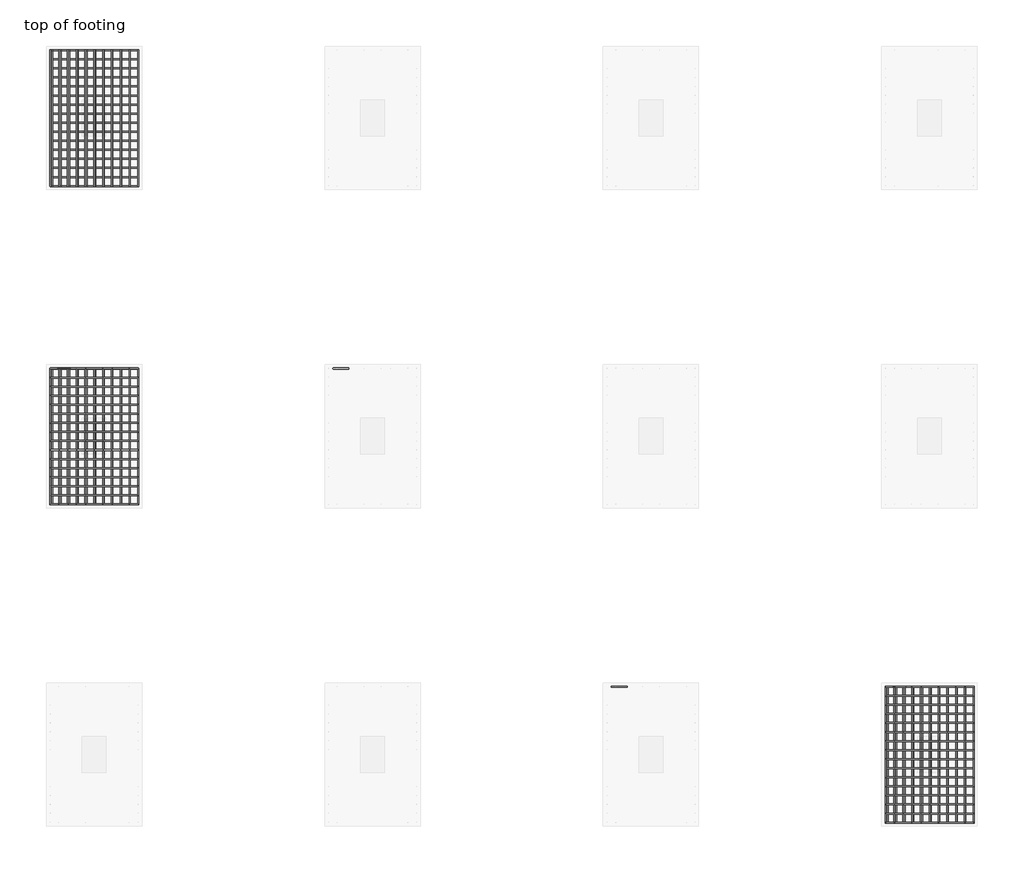
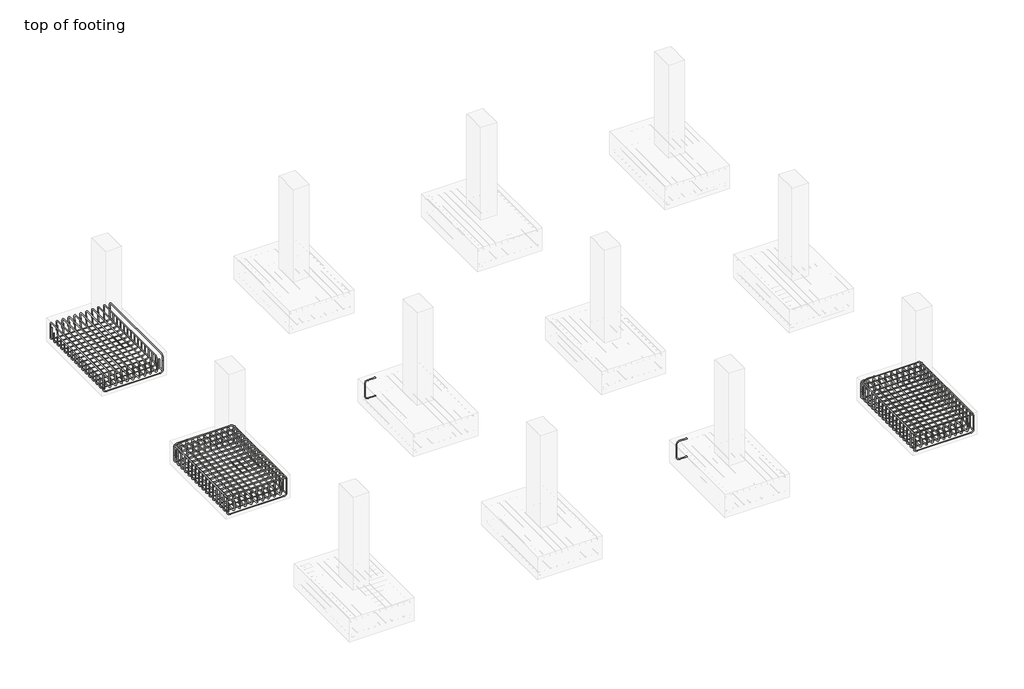
# One storey, part 3 of 8: 15 reinforcing bars.
"""IFC4 building model written with IfcOpenShell, lengths in millimetres."""

from ifc_helpers import new_model, si_unit, point, frame, origin, place, context, project, spatial, polyline, circle_curve, trimmed, segment, composite_curve, source, transform, mapped, element, save
from ifc_brep_helpers import swept_disk

model = new_model("IFC4")

# Units and contexts
model_context = context("Model", 3, world=origin())
ifc_project = project(units=[si_unit("LENGTHUNIT", "METRE", prefix="MILLI")], contexts=[model_context])

# Site, building, storey
site = spatial("IfcSite", under=ifc_project)
building = spatial("IfcBuilding", under=site)
storey = spatial("IfcBuildingStorey", under=building, Name="top of footing", Elevation=-1828.8)

# Reinforcing bars
placement = place(None, origin())
reinforcing_bar_shape = source(origin(), model_context, "Body", "SolidModel", [
    swept_disk(composite_curve([segment(polyline([(-10685.4300189, 12682.8075251, -2014.4920065), (-10685.4300189, 12682.8075251, -2161.7920065)]), True, "CONTINUOUS"), segment(trimmed(circle_curve(frame((-10685.4300189, 12729.1575251, -2161.7920065), z_axis=(1.0, 0.0, 0.0), x_axis=(0.0, -46.350000000000364, 0.0)), 46.35), [point((-10685.4300189, 12682.8075251, -2161.7920065))], [point((-10685.4300189, 12729.1575251, -2208.1420065))], True, "CARTESIAN"), True, "CONTINUOUS"), segment(polyline([(-10685.4300189, 12729.1575251, -2208.1420065), (-10685.4300189, 14343.7575251, -2208.1420065)]), True, "CONTINUOUS"), segment(trimmed(circle_curve(frame((-10685.4300189, 14343.7575251, -2161.7920065), z_axis=(1.0, 0.0, 0.0), x_axis=(0.0, 0.0, -46.350000000000364)), 46.35), [point((-10685.4300189, 14343.7575251, -2208.1420065))], [point((-10685.4300189, 14390.1075251, -2161.7920065))], True, "CARTESIAN"), True, "CONTINUOUS"), segment(polyline([(-10685.4300189, 14390.1075251, -2161.7920065), (-10685.4300189, 14390.1075251, -2014.4920065)]), True, "CONTINUOUS")], self_intersect=False), 6.35),
])
element("IfcReinforcingBar", 1, at=placement, inside=storey, context=model_context, shape_type="MappedRepresentation", body=[
    mapped(reinforcing_bar_shape, transform((0.0, 0.0, 0.0), x_axis=(1.0, 0.0, 0.0), y_axis=(0.0, 1.0, 0.0), z_axis=(0.0, 0.0, 1.0))),
    mapped(reinforcing_bar_shape, transform((-108.3645139, 0.0, 0.0), x_axis=(1.0, 0.0, 0.0), y_axis=(0.0, 1.0, 0.0), z_axis=(0.0, 0.0, 1.0))),
    mapped(reinforcing_bar_shape, transform((-216.7290279, 0.0, 0.0), x_axis=(1.0, 0.0, 0.0), y_axis=(0.0, 1.0, 0.0), z_axis=(0.0, 0.0, 1.0))),
    mapped(reinforcing_bar_shape, transform((-325.0935418, 0.0, 0.0), x_axis=(1.0, 0.0, 0.0), y_axis=(0.0, 1.0, 0.0), z_axis=(0.0, 0.0, 1.0))),
    mapped(reinforcing_bar_shape, transform((-433.4580557, 0.0, 0.0), x_axis=(1.0, 0.0, 0.0), y_axis=(0.0, 1.0, 0.0), z_axis=(0.0, 0.0, 1.0))),
    mapped(reinforcing_bar_shape, transform((-541.8225696, 0.0, 0.0), x_axis=(1.0, 0.0, 0.0), y_axis=(0.0, 1.0, 0.0), z_axis=(0.0, 0.0, 1.0))),
    mapped(reinforcing_bar_shape, transform((-650.1870836, 0.0, 0.0), x_axis=(1.0, 0.0, 0.0), y_axis=(0.0, 1.0, 0.0), z_axis=(0.0, 0.0, 1.0))),
    mapped(reinforcing_bar_shape, transform((-758.5515975, 0.0, 0.0), x_axis=(1.0, 0.0, 0.0), y_axis=(0.0, 1.0, 0.0), z_axis=(0.0, 0.0, 1.0))),
    mapped(reinforcing_bar_shape, transform((-866.9161114, 0.0, 0.0), x_axis=(1.0, 0.0, 0.0), y_axis=(0.0, 1.0, 0.0), z_axis=(0.0, 0.0, 1.0))),
    mapped(reinforcing_bar_shape, transform((-975.2806253, 0.0, 0.0), x_axis=(1.0, 0.0, 0.0), y_axis=(0.0, 1.0, 0.0), z_axis=(0.0, 0.0, 1.0))),
    mapped(reinforcing_bar_shape, transform((-1083.6451393, 0.0, 0.0), x_axis=(1.0, 0.0, 0.0), y_axis=(0.0, 1.0, 0.0), z_axis=(0.0, 0.0, 1.0))),
])
reinforcing_bar_2_shape = source(origin(), model_context, "Body", "SolidModel", [
    swept_disk(composite_curve([segment(polyline([(-11792.7300189, 12682.8075251, -2085.8010212), (-11792.7300189, 12682.8075251, -1938.5010212)]), True, "CONTINUOUS"), segment(trimmed(circle_curve(frame((-11792.7300189, 12729.1575251, -1938.5010212), z_axis=(-1.0, 0.0, 0.0), x_axis=(0.0, -46.350000000000364, 0.0)), 46.35), [point((-11792.7300189, 12682.8075251, -1938.5010212))], [point((-11792.7300189, 12729.1575251, -1892.1510212))], True, "CARTESIAN"), True, "CONTINUOUS"), segment(polyline([(-11792.7300189, 12729.1575251, -1892.1510212), (-11792.7300189, 14343.7575251, -1892.1510212)]), True, "CONTINUOUS"), segment(trimmed(circle_curve(frame((-11792.7300189, 14343.7575251, -1938.5010212), z_axis=(-1.0, 0.0, 0.0), x_axis=(0.0, 0.0, 46.34999999999991)), 46.35), [point((-11792.7300189, 14343.7575251, -1892.1510212))], [point((-11792.7300189, 14390.1075251, -1938.5010212))], True, "CARTESIAN"), True, "CONTINUOUS"), segment(polyline([(-11792.7300189, 14390.1075251, -1938.5010212), (-11792.7300189, 14390.1075251, -2085.8010212)]), True, "CONTINUOUS")], self_intersect=False), 6.35),
])
element("IfcReinforcingBar", 2, at=placement, inside=storey, context=model_context, shape_type="MappedRepresentation", body=[
    mapped(reinforcing_bar_2_shape, transform((0.0, 0.0, 0.0), x_axis=(1.0, 0.0, 0.0), y_axis=(0.0, 1.0, 0.0), z_axis=(0.0, 0.0, 1.0))),
    mapped(reinforcing_bar_2_shape, transform((110.73, 0.0, 0.0), x_axis=(1.0, 0.0, 0.0), y_axis=(0.0, 1.0, 0.0), z_axis=(0.0, 0.0, 1.0))),
    mapped(reinforcing_bar_2_shape, transform((221.46, 0.0, 0.0), x_axis=(1.0, 0.0, 0.0), y_axis=(0.0, 1.0, 0.0), z_axis=(0.0, 0.0, 1.0))),
    mapped(reinforcing_bar_2_shape, transform((332.19, 0.0, 0.0), x_axis=(1.0, 0.0, 0.0), y_axis=(0.0, 1.0, 0.0), z_axis=(0.0, 0.0, 1.0))),
    mapped(reinforcing_bar_2_shape, transform((442.92, 0.0, 0.0), x_axis=(1.0, 0.0, 0.0), y_axis=(0.0, 1.0, 0.0), z_axis=(0.0, 0.0, 1.0))),
    mapped(reinforcing_bar_2_shape, transform((553.65, 0.0, 0.0), x_axis=(1.0, 0.0, 0.0), y_axis=(0.0, 1.0, 0.0), z_axis=(0.0, 0.0, 1.0))),
    mapped(reinforcing_bar_2_shape, transform((664.38, 0.0, 0.0), x_axis=(1.0, 0.0, 0.0), y_axis=(0.0, 1.0, 0.0), z_axis=(0.0, 0.0, 1.0))),
    mapped(reinforcing_bar_2_shape, transform((775.11, 0.0, 0.0), x_axis=(1.0, 0.0, 0.0), y_axis=(0.0, 1.0, 0.0), z_axis=(0.0, 0.0, 1.0))),
    mapped(reinforcing_bar_2_shape, transform((885.84, 0.0, 0.0), x_axis=(1.0, 0.0, 0.0), y_axis=(0.0, 1.0, 0.0), z_axis=(0.0, 0.0, 1.0))),
    mapped(reinforcing_bar_2_shape, transform((996.57, 0.0, 0.0), x_axis=(1.0, 0.0, 0.0), y_axis=(0.0, 1.0, 0.0), z_axis=(0.0, 0.0, 1.0))),
    mapped(reinforcing_bar_2_shape, transform((1107.3, 0.0, 0.0), x_axis=(1.0, 0.0, 0.0), y_axis=(0.0, 1.0, 0.0), z_axis=(0.0, 0.0, 1.0))),
])
reinforcing_bar_3_shape = source(origin(), model_context, "Body", "SolidModel", [
    swept_disk(composite_curve([segment(polyline([(-10685.4300189, 14390.1075251, -2044.8290141), (-10685.4300189, 14390.1075251, -2192.1290141)]), True, "CONTINUOUS"), segment(trimmed(circle_curve(frame((-10731.7800189, 14390.1075251, -2192.1290141), z_axis=(0.0, 1.0, 0.0), x_axis=(46.350000000000364, 0.0, 0.0)), 46.35), [point((-10685.4300189, 14390.1075251, -2192.1290141))], [point((-10731.7800189, 14390.1075251, -2238.4790141))], True, "CARTESIAN"), True, "CONTINUOUS"), segment(polyline([(-10731.7800189, 14390.1075251, -2238.4790141), (-11746.3800189, 14390.1075251, -2238.4790141)]), True, "CONTINUOUS"), segment(trimmed(circle_curve(frame((-11746.3800189, 14390.1075251, -2192.1290141), z_axis=(0.0, 1.0, 0.0), x_axis=(0.0, 0.0, -46.34999999999991)), 46.35), [point((-11746.3800189, 14390.1075251, -2238.4790141))], [point((-11792.7300189, 14390.1075251, -2192.1290141))], True, "CARTESIAN"), True, "CONTINUOUS"), segment(polyline([(-11792.7300189, 14390.1075251, -2192.1290141), (-11792.7300189, 14390.1075251, -2044.8290141)]), True, "CONTINUOUS")], self_intersect=False), 6.35),
])
element("IfcReinforcingBar", 3, at=placement, inside=storey, context=model_context, shape_type="MappedRepresentation", body=[
    mapped(reinforcing_bar_3_shape, transform((0.0, 0.0, 0.0), x_axis=(1.0, 0.0, 0.0), y_axis=(0.0, 1.0, 0.0), z_axis=(0.0, 0.0, 1.0))),
    mapped(reinforcing_bar_3_shape, transform((0.0, -113.82, 0.0), x_axis=(1.0, 0.0, 0.0), y_axis=(0.0, 1.0, 0.0), z_axis=(0.0, 0.0, 1.0))),
    mapped(reinforcing_bar_3_shape, transform((0.0, -227.64, 0.0), x_axis=(1.0, 0.0, 0.0), y_axis=(0.0, 1.0, 0.0), z_axis=(0.0, 0.0, 1.0))),
    mapped(reinforcing_bar_3_shape, transform((0.0, -341.46, 0.0), x_axis=(1.0, 0.0, 0.0), y_axis=(0.0, 1.0, 0.0), z_axis=(0.0, 0.0, 1.0))),
    mapped(reinforcing_bar_3_shape, transform((0.0, -455.28, 0.0), x_axis=(1.0, 0.0, 0.0), y_axis=(0.0, 1.0, 0.0), z_axis=(0.0, 0.0, 1.0))),
    mapped(reinforcing_bar_3_shape, transform((0.0, -569.1, 0.0), x_axis=(1.0, 0.0, 0.0), y_axis=(0.0, 1.0, 0.0), z_axis=(0.0, 0.0, 1.0))),
    mapped(reinforcing_bar_3_shape, transform((0.0, -682.92, 0.0), x_axis=(1.0, 0.0, 0.0), y_axis=(0.0, 1.0, 0.0), z_axis=(0.0, 0.0, 1.0))),
    mapped(reinforcing_bar_3_shape, transform((0.0, -796.74, 0.0), x_axis=(1.0, 0.0, 0.0), y_axis=(0.0, 1.0, 0.0), z_axis=(0.0, 0.0, 1.0))),
    mapped(reinforcing_bar_3_shape, transform((0.0, -910.56, 0.0), x_axis=(1.0, 0.0, 0.0), y_axis=(0.0, 1.0, 0.0), z_axis=(0.0, 0.0, 1.0))),
    mapped(reinforcing_bar_3_shape, transform((0.0, -1024.38, 0.0), x_axis=(1.0, 0.0, 0.0), y_axis=(0.0, 1.0, 0.0), z_axis=(0.0, 0.0, 1.0))),
    mapped(reinforcing_bar_3_shape, transform((0.0, -1138.2, 0.0), x_axis=(1.0, 0.0, 0.0), y_axis=(0.0, 1.0, 0.0), z_axis=(0.0, 0.0, 1.0))),
    mapped(reinforcing_bar_3_shape, transform((0.0, -1252.02, 0.0), x_axis=(1.0, 0.0, 0.0), y_axis=(0.0, 1.0, 0.0), z_axis=(0.0, 0.0, 1.0))),
    mapped(reinforcing_bar_3_shape, transform((0.0, -1365.84, 0.0), x_axis=(1.0, 0.0, 0.0), y_axis=(0.0, 1.0, 0.0), z_axis=(0.0, 0.0, 1.0))),
    mapped(reinforcing_bar_3_shape, transform((0.0, -1479.66, 0.0), x_axis=(1.0, 0.0, 0.0), y_axis=(0.0, 1.0, 0.0), z_axis=(0.0, 0.0, 1.0))),
    mapped(reinforcing_bar_3_shape, transform((0.0, -1593.48, 0.0), x_axis=(1.0, 0.0, 0.0), y_axis=(0.0, 1.0, 0.0), z_axis=(0.0, 0.0, 1.0))),
    mapped(reinforcing_bar_3_shape, transform((0.0, -1707.3, 0.0), x_axis=(1.0, 0.0, 0.0), y_axis=(0.0, 1.0, 0.0), z_axis=(0.0, 0.0, 1.0))),
])
reinforcing_bar_4_shape = source(origin(), model_context, "Body", "SolidModel", [
    swept_disk(composite_curve([segment(polyline([(-10685.4300189, 8682.8075251, -2014.4920065), (-10685.4300189, 8682.8075251, -2161.7920065)]), True, "CONTINUOUS"), segment(trimmed(circle_curve(frame((-10685.4300189, 8729.1575251, -2161.7920065), z_axis=(1.0, 0.0, 0.0), x_axis=(0.0, -46.350000000000364, 0.0)), 46.35), [point((-10685.4300189, 8682.8075251, -2161.7920065))], [point((-10685.4300189, 8729.1575251, -2208.1420065))], True, "CARTESIAN"), True, "CONTINUOUS"), segment(polyline([(-10685.4300189, 8729.1575251, -2208.1420065), (-10685.4300189, 10343.7575251, -2208.1420065)]), True, "CONTINUOUS"), segment(trimmed(circle_curve(frame((-10685.4300189, 10343.7575251, -2161.7920065), z_axis=(1.0, 0.0, 0.0), x_axis=(0.0, 0.0, -46.350000000000364)), 46.35), [point((-10685.4300189, 10343.7575251, -2208.1420065))], [point((-10685.4300189, 10390.1075251, -2161.7920065))], True, "CARTESIAN"), True, "CONTINUOUS"), segment(polyline([(-10685.4300189, 10390.1075251, -2161.7920065), (-10685.4300189, 10390.1075251, -2014.4920065)]), True, "CONTINUOUS")], self_intersect=False), 6.35),
])
element("IfcReinforcingBar", 4, at=placement, inside=storey, context=model_context, shape_type="MappedRepresentation", body=[
    mapped(reinforcing_bar_4_shape, transform((0.0, 0.0, 0.0), x_axis=(1.0, 0.0, 0.0), y_axis=(0.0, 1.0, 0.0), z_axis=(0.0, 0.0, 1.0))),
    mapped(reinforcing_bar_4_shape, transform((-108.3645139, 0.0, 0.0), x_axis=(1.0, 0.0, 0.0), y_axis=(0.0, 1.0, 0.0), z_axis=(0.0, 0.0, 1.0))),
    mapped(reinforcing_bar_4_shape, transform((-216.7290279, 0.0, 0.0), x_axis=(1.0, 0.0, 0.0), y_axis=(0.0, 1.0, 0.0), z_axis=(0.0, 0.0, 1.0))),
    mapped(reinforcing_bar_4_shape, transform((-325.0935418, 0.0, 0.0), x_axis=(1.0, 0.0, 0.0), y_axis=(0.0, 1.0, 0.0), z_axis=(0.0, 0.0, 1.0))),
    mapped(reinforcing_bar_4_shape, transform((-433.4580557, 0.0, 0.0), x_axis=(1.0, 0.0, 0.0), y_axis=(0.0, 1.0, 0.0), z_axis=(0.0, 0.0, 1.0))),
    mapped(reinforcing_bar_4_shape, transform((-541.8225696, 0.0, 0.0), x_axis=(1.0, 0.0, 0.0), y_axis=(0.0, 1.0, 0.0), z_axis=(0.0, 0.0, 1.0))),
    mapped(reinforcing_bar_4_shape, transform((-650.1870836, 0.0, 0.0), x_axis=(1.0, 0.0, 0.0), y_axis=(0.0, 1.0, 0.0), z_axis=(0.0, 0.0, 1.0))),
    mapped(reinforcing_bar_4_shape, transform((-758.5515975, 0.0, 0.0), x_axis=(1.0, 0.0, 0.0), y_axis=(0.0, 1.0, 0.0), z_axis=(0.0, 0.0, 1.0))),
    mapped(reinforcing_bar_4_shape, transform((-866.9161114, 0.0, 0.0), x_axis=(1.0, 0.0, 0.0), y_axis=(0.0, 1.0, 0.0), z_axis=(0.0, 0.0, 1.0))),
    mapped(reinforcing_bar_4_shape, transform((-975.2806253, 0.0, 0.0), x_axis=(1.0, 0.0, 0.0), y_axis=(0.0, 1.0, 0.0), z_axis=(0.0, 0.0, 1.0))),
    mapped(reinforcing_bar_4_shape, transform((-1083.6451393, 0.0, 0.0), x_axis=(1.0, 0.0, 0.0), y_axis=(0.0, 1.0, 0.0), z_axis=(0.0, 0.0, 1.0))),
])
reinforcing_bar_5_shape = source(origin(), model_context, "Body", "SolidModel", [
    swept_disk(composite_curve([segment(polyline([(-11792.7300189, 8682.8075251, -2085.8010212), (-11792.7300189, 8682.8075251, -1938.5010212)]), True, "CONTINUOUS"), segment(trimmed(circle_curve(frame((-11792.7300189, 8729.1575251, -1938.5010212), z_axis=(-1.0, 0.0, 0.0), x_axis=(0.0, -46.350000000000364, 0.0)), 46.35), [point((-11792.7300189, 8682.8075251, -1938.5010212))], [point((-11792.7300189, 8729.1575251, -1892.1510212))], True, "CARTESIAN"), True, "CONTINUOUS"), segment(polyline([(-11792.7300189, 8729.1575251, -1892.1510212), (-11792.7300189, 10343.7575251, -1892.1510212)]), True, "CONTINUOUS"), segment(trimmed(circle_curve(frame((-11792.7300189, 10343.7575251, -1938.5010212), z_axis=(-1.0, 0.0, 0.0), x_axis=(0.0, 0.0, 46.34999999999991)), 46.35), [point((-11792.7300189, 10343.7575251, -1892.1510212))], [point((-11792.7300189, 10390.1075251, -1938.5010212))], True, "CARTESIAN"), True, "CONTINUOUS"), segment(polyline([(-11792.7300189, 10390.1075251, -1938.5010212), (-11792.7300189, 10390.1075251, -2085.8010212)]), True, "CONTINUOUS")], self_intersect=False), 6.35),
])
element("IfcReinforcingBar", 5, at=placement, inside=storey, context=model_context, shape_type="MappedRepresentation", body=[
    mapped(reinforcing_bar_5_shape, transform((0.0, 0.0, 0.0), x_axis=(1.0, 0.0, 0.0), y_axis=(0.0, 1.0, 0.0), z_axis=(0.0, 0.0, 1.0))),
    mapped(reinforcing_bar_5_shape, transform((110.73, 0.0, 0.0), x_axis=(1.0, 0.0, 0.0), y_axis=(0.0, 1.0, 0.0), z_axis=(0.0, 0.0, 1.0))),
    mapped(reinforcing_bar_5_shape, transform((221.46, 0.0, 0.0), x_axis=(1.0, 0.0, 0.0), y_axis=(0.0, 1.0, 0.0), z_axis=(0.0, 0.0, 1.0))),
    mapped(reinforcing_bar_5_shape, transform((332.19, 0.0, 0.0), x_axis=(1.0, 0.0, 0.0), y_axis=(0.0, 1.0, 0.0), z_axis=(0.0, 0.0, 1.0))),
    mapped(reinforcing_bar_5_shape, transform((442.92, 0.0, 0.0), x_axis=(1.0, 0.0, 0.0), y_axis=(0.0, 1.0, 0.0), z_axis=(0.0, 0.0, 1.0))),
    mapped(reinforcing_bar_5_shape, transform((553.65, 0.0, 0.0), x_axis=(1.0, 0.0, 0.0), y_axis=(0.0, 1.0, 0.0), z_axis=(0.0, 0.0, 1.0))),
    mapped(reinforcing_bar_5_shape, transform((664.38, 0.0, 0.0), x_axis=(1.0, 0.0, 0.0), y_axis=(0.0, 1.0, 0.0), z_axis=(0.0, 0.0, 1.0))),
    mapped(reinforcing_bar_5_shape, transform((775.11, 0.0, 0.0), x_axis=(1.0, 0.0, 0.0), y_axis=(0.0, 1.0, 0.0), z_axis=(0.0, 0.0, 1.0))),
    mapped(reinforcing_bar_5_shape, transform((885.84, 0.0, 0.0), x_axis=(1.0, 0.0, 0.0), y_axis=(0.0, 1.0, 0.0), z_axis=(0.0, 0.0, 1.0))),
    mapped(reinforcing_bar_5_shape, transform((996.57, 0.0, 0.0), x_axis=(1.0, 0.0, 0.0), y_axis=(0.0, 1.0, 0.0), z_axis=(0.0, 0.0, 1.0))),
    mapped(reinforcing_bar_5_shape, transform((1107.3, 0.0, 0.0), x_axis=(1.0, 0.0, 0.0), y_axis=(0.0, 1.0, 0.0), z_axis=(0.0, 0.0, 1.0))),
])
element("IfcReinforcingBar", 6, at=placement, inside=storey, context=model_context, shape_type="SolidModel", body=[
    swept_disk(composite_curve([segment(polyline([(-11543.0309105, 10390.1075251, -2232.45), (-11690.3309105, 10390.1075251, -2232.45)]), True, "CONTINUOUS"), segment(trimmed(circle_curve(frame((-11690.3309105, 10390.1075251, -2186.1), z_axis=(0.0, 1.0, 0.0), x_axis=(0.0, 0.0, -46.34999999999991)), 46.35), [point((-11690.3309105, 10390.1075251, -2232.45))], [point((-11736.6809105, 10390.1075251, -2186.1))], True, "CARTESIAN"), True, "CONTINUOUS"), segment(polyline([(-11736.6809105, 10390.1075251, -2186.1), (-11736.6809105, 10390.1075251, -1921.5)]), True, "CONTINUOUS"), segment(trimmed(circle_curve(frame((-11690.3309105, 10390.1075251, -1921.5), z_axis=(0.0, 1.0, 0.0), x_axis=(-46.349999999998545, 0.0, 0.0)), 46.35), [point((-11736.6809105, 10390.1075251, -1921.5))], [point((-11690.3309105, 10390.1075251, -1875.15))], True, "CARTESIAN"), True, "CONTINUOUS"), segment(polyline([(-11690.3309105, 10390.1075251, -1875.15), (-11543.0309105, 10390.1075251, -1875.15)]), True, "CONTINUOUS")], self_intersect=False), 6.35),
])
reinforcing_bar_6_shape = source(origin(), model_context, "Body", "SolidModel", [
    swept_disk(composite_curve([segment(polyline([(-10685.4300189, 10390.1075251, -2044.8290141), (-10685.4300189, 10390.1075251, -2192.1290141)]), True, "CONTINUOUS"), segment(trimmed(circle_curve(frame((-10731.7800189, 10390.1075251, -2192.1290141), z_axis=(0.0, 1.0, 0.0), x_axis=(46.350000000000364, 0.0, 0.0)), 46.35), [point((-10685.4300189, 10390.1075251, -2192.1290141))], [point((-10731.7800189, 10390.1075251, -2238.4790141))], True, "CARTESIAN"), True, "CONTINUOUS"), segment(polyline([(-10731.7800189, 10390.1075251, -2238.4790141), (-11746.3800189, 10390.1075251, -2238.4790141)]), True, "CONTINUOUS"), segment(trimmed(circle_curve(frame((-11746.3800189, 10390.1075251, -2192.1290141), z_axis=(0.0, 1.0, 0.0), x_axis=(0.0, 0.0, -46.34999999999991)), 46.35), [point((-11746.3800189, 10390.1075251, -2238.4790141))], [point((-11792.7300189, 10390.1075251, -2192.1290141))], True, "CARTESIAN"), True, "CONTINUOUS"), segment(polyline([(-11792.7300189, 10390.1075251, -2192.1290141), (-11792.7300189, 10390.1075251, -2044.8290141)]), True, "CONTINUOUS")], self_intersect=False), 6.35),
])
element("IfcReinforcingBar", 7, at=placement, inside=storey, context=model_context, shape_type="MappedRepresentation", body=[
    mapped(reinforcing_bar_6_shape, transform((0.0, 0.0, 0.0), x_axis=(1.0, 0.0, 0.0), y_axis=(0.0, 1.0, 0.0), z_axis=(0.0, 0.0, 1.0))),
    mapped(reinforcing_bar_6_shape, transform((0.0, -113.82, 0.0), x_axis=(1.0, 0.0, 0.0), y_axis=(0.0, 1.0, 0.0), z_axis=(0.0, 0.0, 1.0))),
    mapped(reinforcing_bar_6_shape, transform((0.0, -227.64, 0.0), x_axis=(1.0, 0.0, 0.0), y_axis=(0.0, 1.0, 0.0), z_axis=(0.0, 0.0, 1.0))),
    mapped(reinforcing_bar_6_shape, transform((0.0, -341.46, 0.0), x_axis=(1.0, 0.0, 0.0), y_axis=(0.0, 1.0, 0.0), z_axis=(0.0, 0.0, 1.0))),
    mapped(reinforcing_bar_6_shape, transform((0.0, -455.28, 0.0), x_axis=(1.0, 0.0, 0.0), y_axis=(0.0, 1.0, 0.0), z_axis=(0.0, 0.0, 1.0))),
    mapped(reinforcing_bar_6_shape, transform((0.0, -569.1, 0.0), x_axis=(1.0, 0.0, 0.0), y_axis=(0.0, 1.0, 0.0), z_axis=(0.0, 0.0, 1.0))),
    mapped(reinforcing_bar_6_shape, transform((0.0, -682.92, 0.0), x_axis=(1.0, 0.0, 0.0), y_axis=(0.0, 1.0, 0.0), z_axis=(0.0, 0.0, 1.0))),
    mapped(reinforcing_bar_6_shape, transform((0.0, -796.74, 0.0), x_axis=(1.0, 0.0, 0.0), y_axis=(0.0, 1.0, 0.0), z_axis=(0.0, 0.0, 1.0))),
    mapped(reinforcing_bar_6_shape, transform((0.0, -910.56, 0.0), x_axis=(1.0, 0.0, 0.0), y_axis=(0.0, 1.0, 0.0), z_axis=(0.0, 0.0, 1.0))),
    mapped(reinforcing_bar_6_shape, transform((0.0, -1024.38, 0.0), x_axis=(1.0, 0.0, 0.0), y_axis=(0.0, 1.0, 0.0), z_axis=(0.0, 0.0, 1.0))),
    mapped(reinforcing_bar_6_shape, transform((0.0, -1138.2, 0.0), x_axis=(1.0, 0.0, 0.0), y_axis=(0.0, 1.0, 0.0), z_axis=(0.0, 0.0, 1.0))),
    mapped(reinforcing_bar_6_shape, transform((0.0, -1252.02, 0.0), x_axis=(1.0, 0.0, 0.0), y_axis=(0.0, 1.0, 0.0), z_axis=(0.0, 0.0, 1.0))),
    mapped(reinforcing_bar_6_shape, transform((0.0, -1365.84, 0.0), x_axis=(1.0, 0.0, 0.0), y_axis=(0.0, 1.0, 0.0), z_axis=(0.0, 0.0, 1.0))),
    mapped(reinforcing_bar_6_shape, transform((0.0, -1479.66, 0.0), x_axis=(1.0, 0.0, 0.0), y_axis=(0.0, 1.0, 0.0), z_axis=(0.0, 0.0, 1.0))),
    mapped(reinforcing_bar_6_shape, transform((0.0, -1593.48, 0.0), x_axis=(1.0, 0.0, 0.0), y_axis=(0.0, 1.0, 0.0), z_axis=(0.0, 0.0, 1.0))),
    mapped(reinforcing_bar_6_shape, transform((0.0, -1707.3, 0.0), x_axis=(1.0, 0.0, 0.0), y_axis=(0.0, 1.0, 0.0), z_axis=(0.0, 0.0, 1.0))),
])
reinforcing_bar_7_shape = source(origin(), model_context, "Body", "SolidModel", [
    swept_disk(composite_curve([segment(polyline([(-11792.7300189, 10390.1075251, -2075.0801535), (-11792.7300189, 10390.1075251, -1927.7801535)]), True, "CONTINUOUS"), segment(trimmed(circle_curve(frame((-11746.3800189, 10390.1075251, -1927.7801535), z_axis=(0.0, 1.0, 0.0), x_axis=(-46.350000000000364, 0.0, 0.0)), 46.35), [point((-11792.7300189, 10390.1075251, -1927.7801535))], [point((-11746.3800189, 10390.1075251, -1881.4301535))], True, "CARTESIAN"), True, "CONTINUOUS"), segment(polyline([(-11746.3800189, 10390.1075251, -1881.4301535), (-10731.7800189, 10390.1075251, -1881.4301535)]), True, "CONTINUOUS"), segment(trimmed(circle_curve(frame((-10731.7800189, 10390.1075251, -1927.7801535), z_axis=(0.0, 1.0, 0.0), x_axis=(0.0, 0.0, 46.350000000000136)), 46.35), [point((-10731.7800189, 10390.1075251, -1881.4301535))], [point((-10685.4300189, 10390.1075251, -1927.7801535))], True, "CARTESIAN"), True, "CONTINUOUS"), segment(polyline([(-10685.4300189, 10390.1075251, -1927.7801535), (-10685.4300189, 10390.1075251, -2075.0801535)]), True, "CONTINUOUS")], self_intersect=False), 6.35),
])
element("IfcReinforcingBar", 8, at=placement, inside=storey, context=model_context, shape_type="MappedRepresentation", body=[
    mapped(reinforcing_bar_7_shape, transform((0.0, 0.0, 0.0), x_axis=(1.0, 0.0, 0.0), y_axis=(0.0, 1.0, 0.0), z_axis=(0.0, 0.0, 1.0))),
    mapped(reinforcing_bar_7_shape, transform((0.0, -113.82, 0.0), x_axis=(1.0, 0.0, 0.0), y_axis=(0.0, 1.0, 0.0), z_axis=(0.0, 0.0, 1.0))),
    mapped(reinforcing_bar_7_shape, transform((0.0, -227.64, 0.0), x_axis=(1.0, 0.0, 0.0), y_axis=(0.0, 1.0, 0.0), z_axis=(0.0, 0.0, 1.0))),
    mapped(reinforcing_bar_7_shape, transform((0.0, -341.46, 0.0), x_axis=(1.0, 0.0, 0.0), y_axis=(0.0, 1.0, 0.0), z_axis=(0.0, 0.0, 1.0))),
    mapped(reinforcing_bar_7_shape, transform((0.0, -455.28, 0.0), x_axis=(1.0, 0.0, 0.0), y_axis=(0.0, 1.0, 0.0), z_axis=(0.0, 0.0, 1.0))),
    mapped(reinforcing_bar_7_shape, transform((0.0, -569.1, 0.0), x_axis=(1.0, 0.0, 0.0), y_axis=(0.0, 1.0, 0.0), z_axis=(0.0, 0.0, 1.0))),
    mapped(reinforcing_bar_7_shape, transform((0.0, -682.92, 0.0), x_axis=(1.0, 0.0, 0.0), y_axis=(0.0, 1.0, 0.0), z_axis=(0.0, 0.0, 1.0))),
    mapped(reinforcing_bar_7_shape, transform((0.0, -796.74, 0.0), x_axis=(1.0, 0.0, 0.0), y_axis=(0.0, 1.0, 0.0), z_axis=(0.0, 0.0, 1.0))),
    mapped(reinforcing_bar_7_shape, transform((0.0, -910.56, 0.0), x_axis=(1.0, 0.0, 0.0), y_axis=(0.0, 1.0, 0.0), z_axis=(0.0, 0.0, 1.0))),
    mapped(reinforcing_bar_7_shape, transform((0.0, -1024.38, 0.0), x_axis=(1.0, 0.0, 0.0), y_axis=(0.0, 1.0, 0.0), z_axis=(0.0, 0.0, 1.0))),
    mapped(reinforcing_bar_7_shape, transform((0.0, -1138.2, 0.0), x_axis=(1.0, 0.0, 0.0), y_axis=(0.0, 1.0, 0.0), z_axis=(0.0, 0.0, 1.0))),
    mapped(reinforcing_bar_7_shape, transform((0.0, -1252.02, 0.0), x_axis=(1.0, 0.0, 0.0), y_axis=(0.0, 1.0, 0.0), z_axis=(0.0, 0.0, 1.0))),
    mapped(reinforcing_bar_7_shape, transform((0.0, -1365.84, 0.0), x_axis=(1.0, 0.0, 0.0), y_axis=(0.0, 1.0, 0.0), z_axis=(0.0, 0.0, 1.0))),
    mapped(reinforcing_bar_7_shape, transform((0.0, -1479.66, 0.0), x_axis=(1.0, 0.0, 0.0), y_axis=(0.0, 1.0, 0.0), z_axis=(0.0, 0.0, 1.0))),
    mapped(reinforcing_bar_7_shape, transform((0.0, -1593.48, 0.0), x_axis=(1.0, 0.0, 0.0), y_axis=(0.0, 1.0, 0.0), z_axis=(0.0, 0.0, 1.0))),
    mapped(reinforcing_bar_7_shape, transform((0.0, -1707.3, 0.0), x_axis=(1.0, 0.0, 0.0), y_axis=(0.0, 1.0, 0.0), z_axis=(0.0, 0.0, 1.0))),
])
element("IfcReinforcingBar", 9, at=placement, inside=storey, context=model_context, shape_type="SolidModel", body=[
    swept_disk(composite_curve([segment(polyline([(-4543.0309105, 6390.1075251, -2232.45), (-4690.3309105, 6390.1075251, -2232.45)]), True, "CONTINUOUS"), segment(trimmed(circle_curve(frame((-4690.3309105, 6390.1075251, -2186.1), z_axis=(0.0, 1.0, 0.0), x_axis=(0.0, 0.0, -46.34999999999991)), 46.35), [point((-4690.3309105, 6390.1075251, -2232.45))], [point((-4736.6809105, 6390.1075251, -2186.1))], True, "CARTESIAN"), True, "CONTINUOUS"), segment(polyline([(-4736.6809105, 6390.1075251, -2186.1), (-4736.6809105, 6390.1075251, -1921.5)]), True, "CONTINUOUS"), segment(trimmed(circle_curve(frame((-4690.3309105, 6390.1075251, -1921.5), z_axis=(0.0, 1.0, 0.0), x_axis=(-46.350000000000364, 0.0, 0.0)), 46.35), [point((-4736.6809105, 6390.1075251, -1921.5))], [point((-4690.3309105, 6390.1075251, -1875.15))], True, "CARTESIAN"), True, "CONTINUOUS"), segment(polyline([(-4690.3309105, 6390.1075251, -1875.15), (-4543.0309105, 6390.1075251, -1875.15)]), True, "CONTINUOUS")], self_intersect=False), 6.35),
])
reinforcing_bar_8_shape = source(origin(), model_context, "Body", "SolidModel", [
    swept_disk(composite_curve([segment(polyline([(-185.4300189, 4682.8075251, -2014.4920065), (-185.4300189, 4682.8075251, -2161.7920065)]), True, "CONTINUOUS"), segment(trimmed(circle_curve(frame((-185.4300189, 4729.1575251, -2161.7920065), z_axis=(1.0, 0.0, 0.0), x_axis=(0.0, -46.350000000000364, 0.0)), 46.35), [point((-185.4300189, 4682.8075251, -2161.7920065))], [point((-185.4300189, 4729.1575251, -2208.1420065))], True, "CARTESIAN"), True, "CONTINUOUS"), segment(polyline([(-185.4300189, 4729.1575251, -2208.1420065), (-185.4300189, 6343.7575251, -2208.1420065)]), True, "CONTINUOUS"), segment(trimmed(circle_curve(frame((-185.4300189, 6343.7575251, -2161.7920065), z_axis=(1.0, 0.0, 0.0), x_axis=(0.0, 0.0, -46.350000000000364)), 46.35), [point((-185.4300189, 6343.7575251, -2208.1420065))], [point((-185.4300189, 6390.1075251, -2161.7920065))], True, "CARTESIAN"), True, "CONTINUOUS"), segment(polyline([(-185.4300189, 6390.1075251, -2161.7920065), (-185.4300189, 6390.1075251, -2014.4920065)]), True, "CONTINUOUS")], self_intersect=False), 6.35),
])
element("IfcReinforcingBar", 10, at=placement, inside=storey, context=model_context, shape_type="MappedRepresentation", body=[
    mapped(reinforcing_bar_8_shape, transform((0.0, 0.0, 0.0), x_axis=(1.0, 0.0, 0.0), y_axis=(0.0, 1.0, 0.0), z_axis=(0.0, 0.0, 1.0))),
    mapped(reinforcing_bar_8_shape, transform((-108.3645139, 0.0, 0.0), x_axis=(1.0, 0.0, 0.0), y_axis=(0.0, 1.0, 0.0), z_axis=(0.0, 0.0, 1.0))),
    mapped(reinforcing_bar_8_shape, transform((-216.7290279, 0.0, 0.0), x_axis=(1.0, 0.0, 0.0), y_axis=(0.0, 1.0, 0.0), z_axis=(0.0, 0.0, 1.0))),
    mapped(reinforcing_bar_8_shape, transform((-325.0935418, 0.0, 0.0), x_axis=(1.0, 0.0, 0.0), y_axis=(0.0, 1.0, 0.0), z_axis=(0.0, 0.0, 1.0))),
    mapped(reinforcing_bar_8_shape, transform((-433.4580557, 0.0, 0.0), x_axis=(1.0, 0.0, 0.0), y_axis=(0.0, 1.0, 0.0), z_axis=(0.0, 0.0, 1.0))),
    mapped(reinforcing_bar_8_shape, transform((-541.8225696, 0.0, 0.0), x_axis=(1.0, 0.0, 0.0), y_axis=(0.0, 1.0, 0.0), z_axis=(0.0, 0.0, 1.0))),
    mapped(reinforcing_bar_8_shape, transform((-650.1870836, 0.0, 0.0), x_axis=(1.0, 0.0, 0.0), y_axis=(0.0, 1.0, 0.0), z_axis=(0.0, 0.0, 1.0))),
    mapped(reinforcing_bar_8_shape, transform((-758.5515975, 0.0, 0.0), x_axis=(1.0, 0.0, 0.0), y_axis=(0.0, 1.0, 0.0), z_axis=(0.0, 0.0, 1.0))),
    mapped(reinforcing_bar_8_shape, transform((-866.9161114, 0.0, 0.0), x_axis=(1.0, 0.0, 0.0), y_axis=(0.0, 1.0, 0.0), z_axis=(0.0, 0.0, 1.0))),
    mapped(reinforcing_bar_8_shape, transform((-975.2806253, 0.0, 0.0), x_axis=(1.0, 0.0, 0.0), y_axis=(0.0, 1.0, 0.0), z_axis=(0.0, 0.0, 1.0))),
    mapped(reinforcing_bar_8_shape, transform((-1083.6451393, 0.0, 0.0), x_axis=(1.0, 0.0, 0.0), y_axis=(0.0, 1.0, 0.0), z_axis=(0.0, 0.0, 1.0))),
])
reinforcing_bar_9_shape = source(origin(), model_context, "Body", "SolidModel", [
    swept_disk(composite_curve([segment(polyline([(-1292.7300189, 4682.8075251, -2085.8010212), (-1292.7300189, 4682.8075251, -1938.5010212)]), True, "CONTINUOUS"), segment(trimmed(circle_curve(frame((-1292.7300189, 4729.1575251, -1938.5010212), z_axis=(-1.0, 0.0, 0.0), x_axis=(0.0, -46.350000000000364, 0.0)), 46.35), [point((-1292.7300189, 4682.8075251, -1938.5010212))], [point((-1292.7300189, 4729.1575251, -1892.1510212))], True, "CARTESIAN"), True, "CONTINUOUS"), segment(polyline([(-1292.7300189, 4729.1575251, -1892.1510212), (-1292.7300189, 6343.7575251, -1892.1510212)]), True, "CONTINUOUS"), segment(trimmed(circle_curve(frame((-1292.7300189, 6343.7575251, -1938.5010212), z_axis=(-1.0, 0.0, 0.0), x_axis=(0.0, 0.0, 46.34999999999991)), 46.35), [point((-1292.7300189, 6343.7575251, -1892.1510212))], [point((-1292.7300189, 6390.1075251, -1938.5010212))], True, "CARTESIAN"), True, "CONTINUOUS"), segment(polyline([(-1292.7300189, 6390.1075251, -1938.5010212), (-1292.7300189, 6390.1075251, -2085.8010212)]), True, "CONTINUOUS")], self_intersect=False), 6.35),
])
element("IfcReinforcingBar", 11, at=placement, inside=storey, context=model_context, shape_type="MappedRepresentation", body=[
    mapped(reinforcing_bar_9_shape, transform((0.0, 0.0, 0.0), x_axis=(1.0, 0.0, 0.0), y_axis=(0.0, 1.0, 0.0), z_axis=(0.0, 0.0, 1.0))),
    mapped(reinforcing_bar_9_shape, transform((110.73, 0.0, 0.0), x_axis=(1.0, 0.0, 0.0), y_axis=(0.0, 1.0, 0.0), z_axis=(0.0, 0.0, 1.0))),
    mapped(reinforcing_bar_9_shape, transform((221.46, 0.0, 0.0), x_axis=(1.0, 0.0, 0.0), y_axis=(0.0, 1.0, 0.0), z_axis=(0.0, 0.0, 1.0))),
    mapped(reinforcing_bar_9_shape, transform((332.19, 0.0, 0.0), x_axis=(1.0, 0.0, 0.0), y_axis=(0.0, 1.0, 0.0), z_axis=(0.0, 0.0, 1.0))),
    mapped(reinforcing_bar_9_shape, transform((442.92, 0.0, 0.0), x_axis=(1.0, 0.0, 0.0), y_axis=(0.0, 1.0, 0.0), z_axis=(0.0, 0.0, 1.0))),
    mapped(reinforcing_bar_9_shape, transform((553.65, 0.0, 0.0), x_axis=(1.0, 0.0, 0.0), y_axis=(0.0, 1.0, 0.0), z_axis=(0.0, 0.0, 1.0))),
    mapped(reinforcing_bar_9_shape, transform((664.38, 0.0, 0.0), x_axis=(1.0, 0.0, 0.0), y_axis=(0.0, 1.0, 0.0), z_axis=(0.0, 0.0, 1.0))),
    mapped(reinforcing_bar_9_shape, transform((775.11, 0.0, 0.0), x_axis=(1.0, 0.0, 0.0), y_axis=(0.0, 1.0, 0.0), z_axis=(0.0, 0.0, 1.0))),
    mapped(reinforcing_bar_9_shape, transform((885.84, 0.0, 0.0), x_axis=(1.0, 0.0, 0.0), y_axis=(0.0, 1.0, 0.0), z_axis=(0.0, 0.0, 1.0))),
    mapped(reinforcing_bar_9_shape, transform((996.57, 0.0, 0.0), x_axis=(1.0, 0.0, 0.0), y_axis=(0.0, 1.0, 0.0), z_axis=(0.0, 0.0, 1.0))),
    mapped(reinforcing_bar_9_shape, transform((1107.3, 0.0, 0.0), x_axis=(1.0, 0.0, 0.0), y_axis=(0.0, 1.0, 0.0), z_axis=(0.0, 0.0, 1.0))),
])
element("IfcReinforcingBar", 12, at=placement, inside=storey, context=model_context, shape_type="SolidModel", body=[
    swept_disk(composite_curve([segment(polyline([(-1043.0309105, 6390.1075251, -2232.45), (-1190.3309105, 6390.1075251, -2232.45)]), True, "CONTINUOUS"), segment(trimmed(circle_curve(frame((-1190.3309105, 6390.1075251, -2186.1), z_axis=(0.0, 1.0, 0.0), x_axis=(0.0, 0.0, -46.34999999999991)), 46.35), [point((-1190.3309105, 6390.1075251, -2232.45))], [point((-1236.6809105, 6390.1075251, -2186.1))], True, "CARTESIAN"), True, "CONTINUOUS"), segment(polyline([(-1236.6809105, 6390.1075251, -2186.1), (-1236.6809105, 6390.1075251, -1921.5)]), True, "CONTINUOUS"), segment(trimmed(circle_curve(frame((-1190.3309105, 6390.1075251, -1921.5), z_axis=(0.0, 1.0, 0.0), x_axis=(-46.34999999999991, 0.0, 0.0)), 46.35), [point((-1236.6809105, 6390.1075251, -1921.5))], [point((-1190.3309105, 6390.1075251, -1875.15))], True, "CARTESIAN"), True, "CONTINUOUS"), segment(polyline([(-1190.3309105, 6390.1075251, -1875.15), (-1043.0309105, 6390.1075251, -1875.15)]), True, "CONTINUOUS")], self_intersect=False), 6.35),
])
reinforcing_bar_10_shape = source(origin(), model_context, "Body", "SolidModel", [
    swept_disk(composite_curve([segment(polyline([(-185.4300189, 6390.1075251, -2044.8290141), (-185.4300189, 6390.1075251, -2192.1290141)]), True, "CONTINUOUS"), segment(trimmed(circle_curve(frame((-231.7800189, 6390.1075251, -2192.1290141), z_axis=(0.0, 1.0, 0.0), x_axis=(46.349999999999994, 0.0, 0.0)), 46.35), [point((-185.4300189, 6390.1075251, -2192.1290141))], [point((-231.7800189, 6390.1075251, -2238.4790141))], True, "CARTESIAN"), True, "CONTINUOUS"), segment(polyline([(-231.7800189, 6390.1075251, -2238.4790141), (-1246.3800189, 6390.1075251, -2238.4790141)]), True, "CONTINUOUS"), segment(trimmed(circle_curve(frame((-1246.3800189, 6390.1075251, -2192.1290141), z_axis=(0.0, 1.0, 0.0), x_axis=(0.0, 0.0, -46.34999999999991)), 46.35), [point((-1246.3800189, 6390.1075251, -2238.4790141))], [point((-1292.7300189, 6390.1075251, -2192.1290141))], True, "CARTESIAN"), True, "CONTINUOUS"), segment(polyline([(-1292.7300189, 6390.1075251, -2192.1290141), (-1292.7300189, 6390.1075251, -2044.8290141)]), True, "CONTINUOUS")], self_intersect=False), 6.35),
])
element("IfcReinforcingBar", 13, at=placement, inside=storey, context=model_context, shape_type="MappedRepresentation", body=[
    mapped(reinforcing_bar_10_shape, transform((0.0, 0.0, 0.0), x_axis=(1.0, 0.0, 0.0), y_axis=(0.0, 1.0, 0.0), z_axis=(0.0, 0.0, 1.0))),
    mapped(reinforcing_bar_10_shape, transform((0.0, -113.82, 0.0), x_axis=(1.0, 0.0, 0.0), y_axis=(0.0, 1.0, 0.0), z_axis=(0.0, 0.0, 1.0))),
    mapped(reinforcing_bar_10_shape, transform((0.0, -227.64, 0.0), x_axis=(1.0, 0.0, 0.0), y_axis=(0.0, 1.0, 0.0), z_axis=(0.0, 0.0, 1.0))),
    mapped(reinforcing_bar_10_shape, transform((0.0, -341.46, 0.0), x_axis=(1.0, 0.0, 0.0), y_axis=(0.0, 1.0, 0.0), z_axis=(0.0, 0.0, 1.0))),
    mapped(reinforcing_bar_10_shape, transform((0.0, -455.28, 0.0), x_axis=(1.0, 0.0, 0.0), y_axis=(0.0, 1.0, 0.0), z_axis=(0.0, 0.0, 1.0))),
    mapped(reinforcing_bar_10_shape, transform((0.0, -569.1, 0.0), x_axis=(1.0, 0.0, 0.0), y_axis=(0.0, 1.0, 0.0), z_axis=(0.0, 0.0, 1.0))),
    mapped(reinforcing_bar_10_shape, transform((0.0, -682.92, 0.0), x_axis=(1.0, 0.0, 0.0), y_axis=(0.0, 1.0, 0.0), z_axis=(0.0, 0.0, 1.0))),
    mapped(reinforcing_bar_10_shape, transform((0.0, -796.74, 0.0), x_axis=(1.0, 0.0, 0.0), y_axis=(0.0, 1.0, 0.0), z_axis=(0.0, 0.0, 1.0))),
    mapped(reinforcing_bar_10_shape, transform((0.0, -910.56, 0.0), x_axis=(1.0, 0.0, 0.0), y_axis=(0.0, 1.0, 0.0), z_axis=(0.0, 0.0, 1.0))),
    mapped(reinforcing_bar_10_shape, transform((0.0, -1024.38, 0.0), x_axis=(1.0, 0.0, 0.0), y_axis=(0.0, 1.0, 0.0), z_axis=(0.0, 0.0, 1.0))),
    mapped(reinforcing_bar_10_shape, transform((0.0, -1138.2, 0.0), x_axis=(1.0, 0.0, 0.0), y_axis=(0.0, 1.0, 0.0), z_axis=(0.0, 0.0, 1.0))),
    mapped(reinforcing_bar_10_shape, transform((0.0, -1252.02, 0.0), x_axis=(1.0, 0.0, 0.0), y_axis=(0.0, 1.0, 0.0), z_axis=(0.0, 0.0, 1.0))),
    mapped(reinforcing_bar_10_shape, transform((0.0, -1365.84, 0.0), x_axis=(1.0, 0.0, 0.0), y_axis=(0.0, 1.0, 0.0), z_axis=(0.0, 0.0, 1.0))),
    mapped(reinforcing_bar_10_shape, transform((0.0, -1479.66, 0.0), x_axis=(1.0, 0.0, 0.0), y_axis=(0.0, 1.0, 0.0), z_axis=(0.0, 0.0, 1.0))),
    mapped(reinforcing_bar_10_shape, transform((0.0, -1593.48, 0.0), x_axis=(1.0, 0.0, 0.0), y_axis=(0.0, 1.0, 0.0), z_axis=(0.0, 0.0, 1.0))),
    mapped(reinforcing_bar_10_shape, transform((0.0, -1707.3, 0.0), x_axis=(1.0, 0.0, 0.0), y_axis=(0.0, 1.0, 0.0), z_axis=(0.0, 0.0, 1.0))),
])
reinforcing_bar_11_shape = source(origin(), model_context, "Body", "SolidModel", [
    swept_disk(composite_curve([segment(polyline([(-1292.7300189, 6390.1075251, -2075.0801535), (-1292.7300189, 6390.1075251, -1927.7801535)]), True, "CONTINUOUS"), segment(trimmed(circle_curve(frame((-1246.3800189, 6390.1075251, -1927.7801535), z_axis=(0.0, 1.0, 0.0), x_axis=(-46.34999999999991, 0.0, 0.0)), 46.35), [point((-1292.7300189, 6390.1075251, -1927.7801535))], [point((-1246.3800189, 6390.1075251, -1881.4301535))], True, "CARTESIAN"), True, "CONTINUOUS"), segment(polyline([(-1246.3800189, 6390.1075251, -1881.4301535), (-231.7800189, 6390.1075251, -1881.4301535)]), True, "CONTINUOUS"), segment(trimmed(circle_curve(frame((-231.7800189, 6390.1075251, -1927.7801535), z_axis=(0.0, 1.0, 0.0), x_axis=(0.0, 0.0, 46.350000000000136)), 46.35), [point((-231.7800189, 6390.1075251, -1881.4301535))], [point((-185.4300189, 6390.1075251, -1927.7801535))], True, "CARTESIAN"), True, "CONTINUOUS"), segment(polyline([(-185.4300189, 6390.1075251, -1927.7801535), (-185.4300189, 6390.1075251, -2075.0801535)]), True, "CONTINUOUS")], self_intersect=False), 6.35),
])
element("IfcReinforcingBar", 14, at=placement, inside=storey, context=model_context, shape_type="MappedRepresentation", body=[
    mapped(reinforcing_bar_11_shape, transform((0.0, 0.0, 0.0), x_axis=(1.0, 0.0, 0.0), y_axis=(0.0, 1.0, 0.0), z_axis=(0.0, 0.0, 1.0))),
    mapped(reinforcing_bar_11_shape, transform((0.0, -113.82, 0.0), x_axis=(1.0, 0.0, 0.0), y_axis=(0.0, 1.0, 0.0), z_axis=(0.0, 0.0, 1.0))),
    mapped(reinforcing_bar_11_shape, transform((0.0, -227.64, 0.0), x_axis=(1.0, 0.0, 0.0), y_axis=(0.0, 1.0, 0.0), z_axis=(0.0, 0.0, 1.0))),
    mapped(reinforcing_bar_11_shape, transform((0.0, -341.46, 0.0), x_axis=(1.0, 0.0, 0.0), y_axis=(0.0, 1.0, 0.0), z_axis=(0.0, 0.0, 1.0))),
    mapped(reinforcing_bar_11_shape, transform((0.0, -455.28, 0.0), x_axis=(1.0, 0.0, 0.0), y_axis=(0.0, 1.0, 0.0), z_axis=(0.0, 0.0, 1.0))),
    mapped(reinforcing_bar_11_shape, transform((0.0, -569.1, 0.0), x_axis=(1.0, 0.0, 0.0), y_axis=(0.0, 1.0, 0.0), z_axis=(0.0, 0.0, 1.0))),
    mapped(reinforcing_bar_11_shape, transform((0.0, -682.92, 0.0), x_axis=(1.0, 0.0, 0.0), y_axis=(0.0, 1.0, 0.0), z_axis=(0.0, 0.0, 1.0))),
    mapped(reinforcing_bar_11_shape, transform((0.0, -796.74, 0.0), x_axis=(1.0, 0.0, 0.0), y_axis=(0.0, 1.0, 0.0), z_axis=(0.0, 0.0, 1.0))),
    mapped(reinforcing_bar_11_shape, transform((0.0, -910.56, 0.0), x_axis=(1.0, 0.0, 0.0), y_axis=(0.0, 1.0, 0.0), z_axis=(0.0, 0.0, 1.0))),
    mapped(reinforcing_bar_11_shape, transform((0.0, -1024.38, 0.0), x_axis=(1.0, 0.0, 0.0), y_axis=(0.0, 1.0, 0.0), z_axis=(0.0, 0.0, 1.0))),
    mapped(reinforcing_bar_11_shape, transform((0.0, -1138.2, 0.0), x_axis=(1.0, 0.0, 0.0), y_axis=(0.0, 1.0, 0.0), z_axis=(0.0, 0.0, 1.0))),
    mapped(reinforcing_bar_11_shape, transform((0.0, -1252.02, 0.0), x_axis=(1.0, 0.0, 0.0), y_axis=(0.0, 1.0, 0.0), z_axis=(0.0, 0.0, 1.0))),
    mapped(reinforcing_bar_11_shape, transform((0.0, -1365.84, 0.0), x_axis=(1.0, 0.0, 0.0), y_axis=(0.0, 1.0, 0.0), z_axis=(0.0, 0.0, 1.0))),
    mapped(reinforcing_bar_11_shape, transform((0.0, -1479.66, 0.0), x_axis=(1.0, 0.0, 0.0), y_axis=(0.0, 1.0, 0.0), z_axis=(0.0, 0.0, 1.0))),
    mapped(reinforcing_bar_11_shape, transform((0.0, -1593.48, 0.0), x_axis=(1.0, 0.0, 0.0), y_axis=(0.0, 1.0, 0.0), z_axis=(0.0, 0.0, 1.0))),
    mapped(reinforcing_bar_11_shape, transform((0.0, -1707.3, 0.0), x_axis=(1.0, 0.0, 0.0), y_axis=(0.0, 1.0, 0.0), z_axis=(0.0, 0.0, 1.0))),
])
element("IfcReinforcingBar", 15, at=placement, inside=storey, context=model_context, shape_type="SolidModel", body=[
    swept_disk(composite_curve([segment(polyline([(-8043.0309105, 10390.1075251, -2232.45), (-8190.3309105, 10390.1075251, -2232.45)]), True, "CONTINUOUS"), segment(trimmed(circle_curve(frame((-8190.3309105, 10390.1075251, -2186.1), z_axis=(0.0, 1.0, 0.0), x_axis=(0.0, 0.0, -46.34999999999991)), 46.35), [point((-8190.3309105, 10390.1075251, -2232.45))], [point((-8236.6809105, 10390.1075251, -2186.1))], True, "CARTESIAN"), True, "CONTINUOUS"), segment(polyline([(-8236.6809105, 10390.1075251, -2186.1), (-8236.6809105, 10390.1075251, -1921.5)]), True, "CONTINUOUS"), segment(trimmed(circle_curve(frame((-8190.3309105, 10390.1075251, -1921.5), z_axis=(0.0, 1.0, 0.0), x_axis=(-46.349999999999454, 0.0, 0.0)), 46.35), [point((-8236.6809105, 10390.1075251, -1921.5))], [point((-8190.3309105, 10390.1075251, -1875.15))], True, "CARTESIAN"), True, "CONTINUOUS"), segment(polyline([(-8190.3309105, 10390.1075251, -1875.15), (-8043.0309105, 10390.1075251, -1875.15)]), True, "CONTINUOUS")], self_intersect=False), 6.35),
])

save(model, "model.ifc")

# Revit data of these elements
# Elements 1, 2, 3, 4, 5, 6, 7, 8, 9, 10, 11, 12, 13, 14, 15 (IfcReinforcingBar)
#   Phase Created = New Construction
